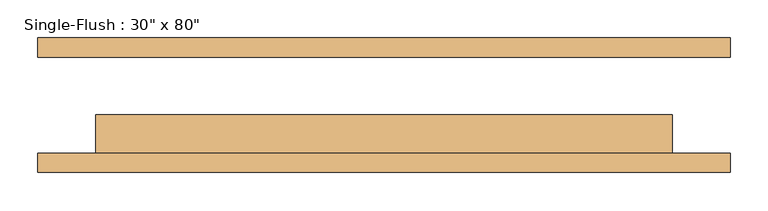
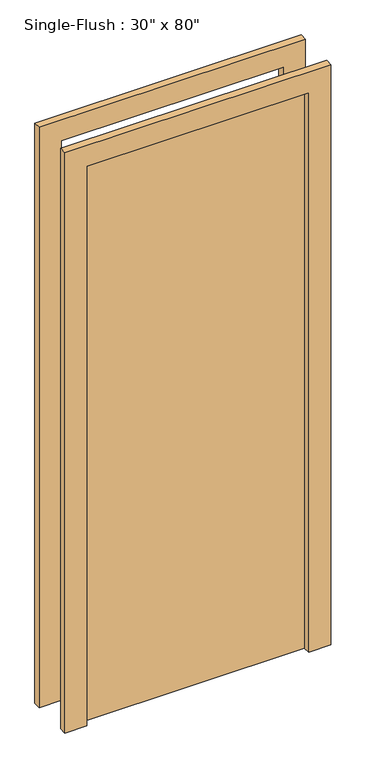
"""IFC4 building model written with IfcOpenShell, lengths in millimetres: door geometry."""

from ifc_helpers import new_model, si_unit, frame, origin, origin_with_axes, place, context, project, spatial, polyline, outline, extrude, source, transform, mapped, element, save


def door_e00f436c(model_context):
    return source(origin(), model_context, "Body", "SweptSolid", [
        extrude(outline(polyline([(2108.2, -457.2), (0.0, -457.2), (0.0, -381.0), (2032.0, -381.0), (2032.0, 381.0), (0.0, 381.0), (0.0, 457.2), (2108.2, 457.2), (2108.2, -457.2)])), frame((0.0, -88.9, 0.0), z_axis=(0.0, 1.0, 0.0), x_axis=(0.0, 0.0, 1.0)), (0.0, 0.0, 1.0), 25.4),
        extrude(outline(polyline([(2108.2, 457.2), (2108.2, -457.2), (0.0, -457.2), (0.0, -381.0), (2032.0, -381.0), (2032.0, 381.0), (0.0, 381.0), (0.0, 457.2), (2108.2, 457.2)])), frame((0.0, 63.5, 0.0), z_axis=(0.0, 1.0, 0.0), x_axis=(0.0, 0.0, 1.0)), (0.0, 0.0, 1.0), 25.4),
        extrude(outline(polyline([(381.0, -12.7), (381.0, -63.5), (-381.0, -63.5), (-381.0, -12.7), (381.0, -12.7)])), origin_with_axes(), (0.0, 0.0, 1.0), 2032.0),
    ])


if __name__ == "__main__":
    model = new_model("IFC4")
    model_context = context("Model", 3, world=origin())
    ifc_project = project(units=[si_unit("LENGTHUNIT", "METRE", prefix="MILLI")], contexts=[model_context])
    site = spatial("IfcSite", under=ifc_project)
    building = spatial("IfcBuilding", under=site)
    placement = place(None, origin())
    door_shape = door_e00f436c(model_context)
    element("IfcDoor", 1, ObjectType="Single-Flush : 30\" x 80\"", at=placement, inside=building, context=model_context, shape_type="MappedRepresentation", body=[
        mapped(door_shape, transform((0.0, 0.0, 0.0), x_axis=(1.0, 0.0, 0.0), y_axis=(0.0, 1.0, 0.0), z_axis=(0.0, 0.0, 1.0))),
    ])
    save(model, "model.ifc")

# Revit data of these elements
# Type "Single-Flush : 30\" x 80\""
#   Type Mark = "5"
#   Assembly Code = "C1020"
#   Thickness = 0' - 2"
#   Height = 6' - 8"
#   Trim Projection Ext = 0' - 1"
#   Trim Projection Int = 0' - 1"
#   Trim Width = 0' - 3"
#   Width = 2' - 6"
#   Door Material = Door - Panel
#   Frame Material = Door - Frame
#   Function = (empty or 0)
#   Wall Closure = (empty or 0)
# Element 1 (IfcDoor, "Single-Flush : 30\" x 80\"")
#   Materials on its faces: "Door - Frame", "Door - Panel"
# Materials
#   "Door - Panel": class "Wood", colour RGB 114 82 51, transparency 0
#   "Door - Frame": colour RGB 153 76 43, transparency 0
